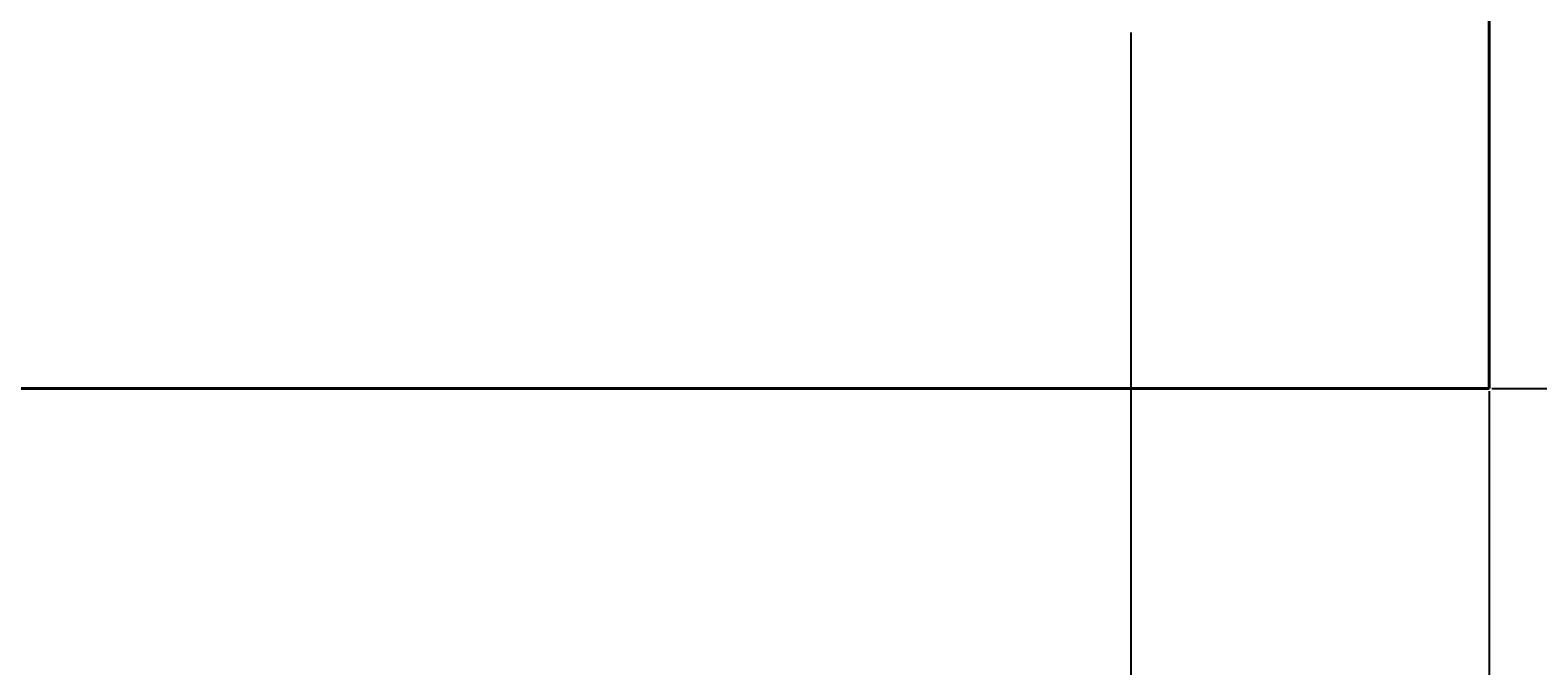
# Model space of a CAD drawing. Units: inches. Extents: x -301 to 715, y -607 to 364.
# Tile 90 of 141: x 96 to 134, y -231 to -215. Entities that reach past the tile are written whole.
import ezdxf

# ---------------------------------------------------------------- set-up
doc = ezdxf.new("R2010")
doc.units = ezdxf.units.IN
doc.header["$MEASUREMENT"] = 0
doc.layers.add('A-ANNO-DIMS', color=2, linetype='Continuous', lineweight=18)
doc.layers.add('A-WALL', color=3, linetype='Continuous', lineweight=40)
doc.styles.get("Standard").update_dxf_attribs({"font": 'arial.ttf'})
doc.dimstyles.get("Standard").update_dxf_attribs({"dimtxt": 0.18, "dimasz": 0.18, "dimexe": 0.18, "dimexo": 0.0625, "dimgap": 0.09, "dimtad": 0, "dimtih": 1, "dimtoh": 1, "dimdec": 1, "dimzin": 0, "dimdsep": 46, "dimlunit": 4, "dimtxsty": 'Standard', "dimcen": 0.09, "dimclrd": 3, "dimclre": 4, "dimclrt": 6, "dimadec": 0, "dimazin": 0, "dimtfac": 1, "dimtdec": 1, "dimtofl": 0, "dimtmove": 0, "dimatfit": 3, "dimfxl": 1, "dimtfill": 2, "dimtfillclr": 51, "dimtolj": 1, "dimtzin": 0, "dimarcsym": 0})

# ---------------------------------------------------------------- blocks, each defined once
blk = doc.blocks.new('*D152')
at = {"layer": 'A-ANNO-DIMS', "color": 4, "lineweight": -2, "transparency": 16777216}
for p, q in [((123.959, -130.818), (233.659, -130.818)), ((132.959, -223.818), (233.659, -223.818))]:
    blk.add_line(p, q, dxfattribs=at)
at = {"layer": 'A-ANNO-DIMS', "color": 3, "lineweight": -2, "transparency": 16777216}
for p, q in [((233.479, -130.998), (233.479, -177.136)), ((233.479, -223.638), (233.479, -177.5))]:
    blk.add_line(p, q, dxfattribs=at)
at = {"layer": 'A-ANNO-DIMS', "color": 3, "transparency": 16777216}
for points in [[(233.449, -130.998), (233.509, -130.998), (233.479, -130.818)], [(233.449, -223.638), (233.509, -223.638), (233.479, -223.818)]]:
    blk.add_solid(points, dxfattribs=at)
at = {"layer": 'Defpoints', "color": 0, "transparency": 16777216}
for p in [(123.897, -130.818), (233.479, -130.818), (132.897, -223.818)]:
    blk.add_point(p, dxfattribs=at)
at = {"layer": 'A-ANNO-DIMS', "color": 6, "transparency": 16777216, "insert": (233.479, -177.318), "char_height": 0.18, "attachment_point": 5, "bg_fill": 1, "box_fill_scale": 1.25, "bg_fill_color": 51, "bg_fill_transparency": 0}
blk.add_mtext('\\A1;7\'-9"', dxfattribs=at)
blk = doc.blocks.new('*D156')
at = {"layer": 'A-ANNO-DIMS', "color": 4, "lineweight": -2, "transparency": 16777216}
for p, q in [((123.897, -214.88), (123.897, -296.865)), ((132.897, -223.88), (132.897, -296.865))]:
    blk.add_line(p, q, dxfattribs=at)
at = {"layer": 'A-ANNO-DIMS', "color": 3, "lineweight": -2, "transparency": 16777216}
for p, q in [((124.077, -296.685), (128.067, -296.685)), ((132.717, -296.685), (128.726, -296.685))]:
    blk.add_line(p, q, dxfattribs=at)
at = {"layer": 'A-ANNO-DIMS', "color": 3, "transparency": 16777216}
for points in [[(124.077, -296.655), (124.077, -296.715), (123.897, -296.685)], [(132.717, -296.655), (132.717, -296.715), (132.897, -296.685)]]:
    blk.add_solid(points, dxfattribs=at)
at = {"layer": 'Defpoints', "color": 0, "transparency": 16777216}
for p in [(123.897, -214.818), (132.897, -223.818), (132.897, -296.685)]:
    blk.add_point(p, dxfattribs=at)
at = {"layer": 'A-ANNO-DIMS', "color": 6, "transparency": 16777216, "insert": (128.397, -296.685), "char_height": 0.18, "attachment_point": 5, "bg_fill": 1, "box_fill_scale": 1.25, "bg_fill_color": 51, "bg_fill_transparency": 0}
blk.add_mtext('\\A1;0\'-9"', dxfattribs=at)

msp = doc.modelspace()

# ---------------------------------------------------------------- linework, layer by layer
at = {"layer": 'A-WALL'}
for p, q in [((132.897, -223.818), (132.897, -124.818)), ((-45.603, -223.818), (132.897, -223.818))]:
    msp.add_line(p, q, dxfattribs=at)

# ---------------------------------------------------------------- dimensions: what is measured, and where the dimension line sits
at = {"layer": 'A-ANNO-DIMS'}
dim = msp.add_linear_dim(base=(233.479, -130.818), p1=(132.897, -223.818), p2=(123.897, -130.818), angle=90, dimstyle='Standard', override={"dimdec": 1, "dimlfac": 1, "dimrnd": 0, "dimzin": 1, "dimdsep": 46, "dimlunit": 4, "dimfrac": 2}, dxfattribs=at)
dim.commit()
dim.dimension.update_dxf_attribs({"geometry": '*D152', "text_midpoint": (233.479, -177.318)})
dim = msp.add_linear_dim(base=(132.897, -296.685), p1=(123.897, -214.818), p2=(132.897, -223.818), dimstyle='Standard', override={"dimdec": 1, "dimlfac": 1, "dimrnd": 0, "dimzin": 1, "dimdsep": 46, "dimlunit": 4, "dimfrac": 2}, dxfattribs=at)
dim.commit()
dim.dimension.update_dxf_attribs({"geometry": '*D156', "text_midpoint": (128.397, -296.685)})

doc.saveas('drawing.dxf')
